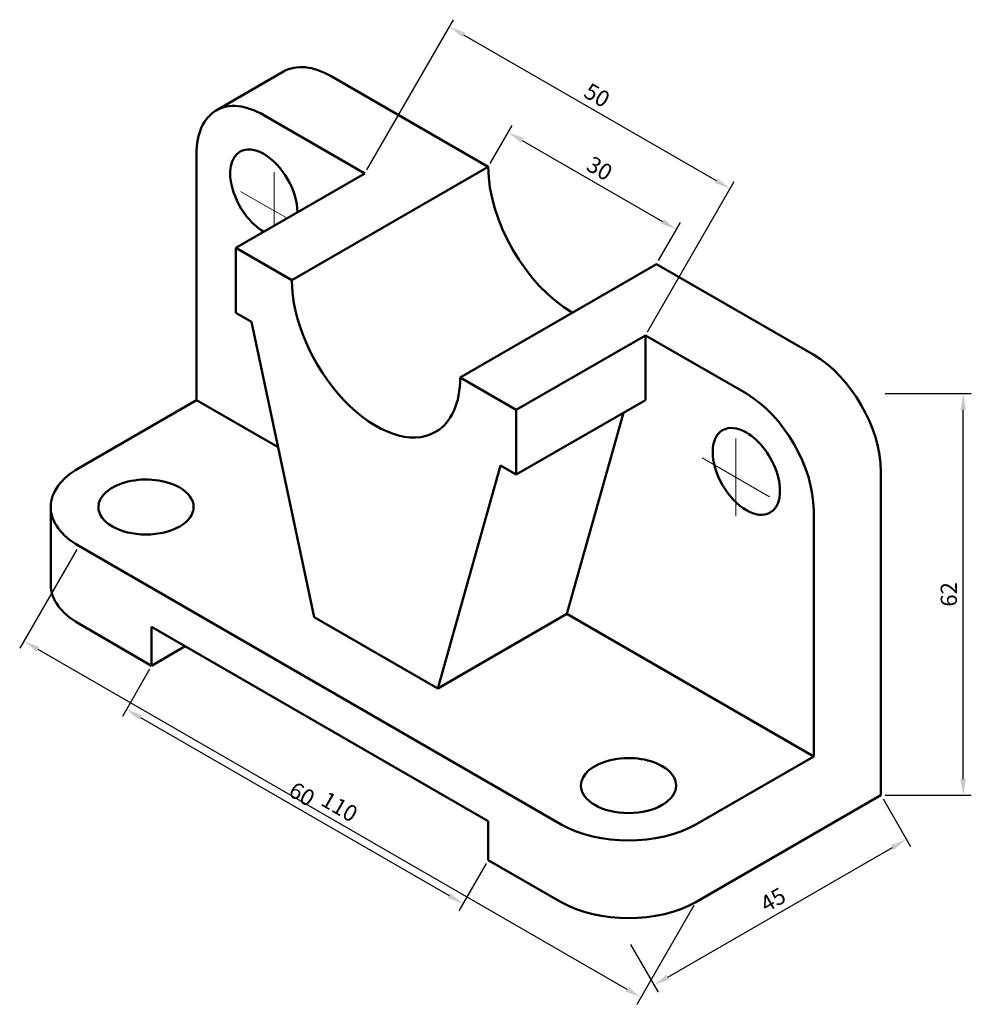
# Model space of a CAD drawing. Units: millimetres. Extents: x 1633 to 1780, y 2750 to 2902.
import ezdxf

# ---------------------------------------------------------------- set-up
doc = ezdxf.new("R2010")
doc.units = ezdxf.units.MM
doc.linetypes.add('CENTER', pattern=[50.8, 31.75, -6.35, 6.35, -6.35])
for name, color, linetype, lineweight in [('M-CNTR', 1, 'CENTER', 18), ('M-DIMS', 2, 'Continuous', 25), ('M-OUTL', 7, 'Continuous', 50)]:
    doc.layers.add(name, color=color, linetype=linetype, lineweight=lineweight)
doc.styles.get("Standard").update_dxf_attribs({"font": 'arial.ttf'})
doc.dimstyles.new('ISO-25', dxfattribs={"dimtxt": 2.5, "dimasz": 2.5, "dimexe": 1.25, "dimexo": 0.625, "dimtad": 1, "dimtxsty": 'Standard', "dimcen": 2.5, "dimadec": 0, "dimazin": 0, "dimtfac": 1, "dimtmove": 0, "dimatfit": 3, "dimfxl": 1, "dimarcsym": 0})

# ---------------------------------------------------------------- blocks, each defined once
blk = doc.blocks.new('*D1')
at = {"layer": 'Defpoints', "color": 0, "transparency": 16777216}
for p in [(1653.65, 2801.94), (1705.61, 2771.94), (1701.72, 2765.19)]:
    blk.add_point(p, dxfattribs=at)
at = {"layer": 'M-DIMS', "color": 0, "lineweight": -2, "transparency": 16777216}
for p, q in [((1653.33, 2801.4), (1649.13, 2794.11)), ((1651.92, 2793.94), (1699.55, 2766.44)), ((1705.3, 2771.4), (1701.09, 2764.11))]:
    blk.add_line(p, q, dxfattribs=at)
at = {"layer": 'M-DIMS', "color": 0, "transparency": 16777216}
for points in [[(1652.13, 2794.31), (1651.71, 2793.58), (1649.75, 2795.19)], [(1699.76, 2766.81), (1699.34, 2766.08), (1701.72, 2765.19)]]:
    blk.add_solid(points, dxfattribs=at)
at = {"layer": 'M-DIMS', "color": 0, "transparency": 16777216, "insert": (1676.69, 2781.84), "char_height": 2.5, "attachment_point": 5, "rotation": 330}
blk.add_mtext('60', dxfattribs=at)
blk = doc.blocks.new('*D2')
at = {"layer": 'Defpoints', "color": 0, "transparency": 16777216}
for p in [(1766.23, 2781.94), (1770.16, 2775.13), (1727.26, 2759.44)]:
    blk.add_point(p, dxfattribs=at)
at = {"layer": 'M-DIMS', "color": 0, "lineweight": -2, "transparency": 16777216}
for p, q in [((1766.54, 2781.4), (1770.78, 2774.05)), ((1733.35, 2753.88), (1767.99, 2773.88)), ((1727.57, 2758.9), (1731.81, 2751.55))]:
    blk.add_line(p, q, dxfattribs=at)
at = {"layer": 'M-DIMS', "color": 0, "transparency": 16777216}
for points in [[(1767.78, 2774.24), (1768.2, 2773.52), (1770.16, 2775.13)], [(1733.14, 2754.24), (1733.56, 2753.52), (1731.19, 2752.63)]]:
    blk.add_solid(points, dxfattribs=at)
at = {"layer": 'M-DIMS', "color": 0, "transparency": 16777216, "insert": (1749.72, 2765.53), "char_height": 2.5, "attachment_point": 5, "rotation": 30}
blk.add_mtext('45', dxfattribs=at)
blk = doc.blocks.new('*D3')
at = {"layer": 'Defpoints', "color": 0, "transparency": 16777216}
for p in [(1766.23, 2843.94), (1778.92, 2843.94), (1766.23, 2781.94)]:
    blk.add_point(p, dxfattribs=at)
at = {"layer": 'M-DIMS', "color": 0, "lineweight": -2, "transparency": 16777216}
for p, q in [((1766.86, 2843.94), (1780.17, 2843.94)), ((1778.92, 2784.44), (1778.92, 2841.44)), ((1766.86, 2781.94), (1780.17, 2781.94))]:
    blk.add_line(p, q, dxfattribs=at)
at = {"layer": 'M-DIMS', "color": 0, "transparency": 16777216}
for points in [[(1778.5, 2841.44), (1779.34, 2841.44), (1778.92, 2843.94)], [(1778.5, 2784.44), (1779.34, 2784.44), (1778.92, 2781.94)]]:
    blk.add_solid(points, dxfattribs=at)
at = {"layer": 'M-DIMS', "color": 0, "transparency": 16777216, "insert": (1777.02, 2812.94), "char_height": 2.5, "attachment_point": 5, "rotation": 90}
blk.add_mtext('62', dxfattribs=at)
blk = doc.blocks.new('*D4')
at = {"layer": 'Defpoints', "color": 0, "transparency": 16777216}
for p in [(1705.61, 2878.94), (1734.67, 2869.28), (1731.59, 2863.94)]:
    blk.add_point(p, dxfattribs=at)
at = {"layer": 'M-DIMS', "color": 0, "lineweight": -2, "transparency": 16777216}
for p, q in [((1705.92, 2879.48), (1709.32, 2885.36)), ((1710.86, 2883.03), (1732.51, 2870.53)), ((1731.9, 2864.48), (1735.3, 2870.36))]:
    blk.add_line(p, q, dxfattribs=at)
at = {"layer": 'M-DIMS', "color": 0, "transparency": 16777216}
for points in [[(1711.07, 2883.39), (1710.65, 2882.67), (1708.69, 2884.28)], [(1732.72, 2870.89), (1732.3, 2870.17), (1734.67, 2869.28)]]:
    blk.add_solid(points, dxfattribs=at)
at = {"layer": 'M-DIMS', "color": 0, "transparency": 16777216, "insert": (1722.63, 2878.43), "char_height": 2.5, "attachment_point": 5, "rotation": 330}
blk.add_mtext('30', dxfattribs=at)
blk = doc.blocks.new('*D5')
at = {"layer": 'Defpoints', "color": 0, "transparency": 16777216}
for p in [(1686.56, 2877.94), (1742.93, 2875.59), (1729.86, 2852.94)]:
    blk.add_point(p, dxfattribs=at)
at = {"layer": 'M-DIMS', "color": 0, "lineweight": -2, "transparency": 16777216}
for p, q in [((1686.87, 2878.48), (1700.26, 2901.67)), ((1701.8, 2899.34), (1740.77, 2876.84)), ((1730.17, 2853.48), (1743.56, 2876.67))]:
    blk.add_line(p, q, dxfattribs=at)
at = {"layer": 'M-DIMS', "color": 0, "transparency": 16777216}
for points in [[(1702.01, 2899.7), (1701.59, 2898.98), (1699.63, 2900.59)], [(1740.98, 2877.2), (1740.56, 2876.48), (1742.93, 2875.59)]]:
    blk.add_solid(points, dxfattribs=at)
at = {"layer": 'M-DIMS', "color": 0, "transparency": 16777216, "insert": (1722.23, 2889.73), "char_height": 2.5, "attachment_point": 5, "rotation": 330}
blk.add_mtext('50', dxfattribs=at)
blk = doc.blocks.new('*D7')
at = {"layer": 'Defpoints', "color": 0, "transparency": 16777216}
for p in [(1642.39, 2820.44), (1737.65, 2765.44), (1729.17, 2750.75)]:
    blk.add_point(p, dxfattribs=at)
at = {"layer": 'M-DIMS', "color": 0, "lineweight": -2, "transparency": 16777216}
for p, q in [((1642.08, 2819.9), (1633.28, 2804.66)), ((1636.07, 2804.5), (1727, 2752)), ((1737.34, 2764.9), (1728.54, 2749.66))]:
    blk.add_line(p, q, dxfattribs=at)
at = {"layer": 'M-DIMS', "color": 0, "transparency": 16777216}
for points in [[(1636.28, 2804.86), (1635.86, 2804.14), (1633.91, 2805.75)], [(1727.21, 2752.36), (1726.8, 2751.64), (1729.17, 2750.75)]]:
    blk.add_solid(points, dxfattribs=at)
at = {"layer": 'M-DIMS', "color": 0, "transparency": 16777216, "insert": (1682.49, 2779.89), "char_height": 2.5, "attachment_point": 5, "rotation": 330}
blk.add_mtext('110', dxfattribs=at)

msp = doc.modelspace()

# ---------------------------------------------------------------- linework, layer by layer
at = {"layer": 'M-CNTR'}
for p, q in [((1672.575, 2872.153), (1672.575, 2878.153)), ((1672.575, 2878.153), (1672.575, 2869.865)), ((1672.575, 2872.153), (1667.379, 2875.153)), ((1667.379, 2875.153), (1674.556, 2871.009)), ((1743.838, 2825.009), (1743.838, 2837.009)), ((1749.034, 2828.009), (1738.642, 2834.009)), ((1743.838, 2831.009), (1749.034, 2828.009)), ((1743.838, 2831.009), (1743.838, 2825.009))]:
    msp.add_line(p, q, dxfattribs=at)
at = {"layer": 'M-OUTL'}
for p, q in [((1663.619, 2887.665), (1674.011, 2893.665)), ((1705.608, 2878.937), (1681.36, 2892.937)), ((1686.556, 2877.937), (1670.967, 2886.937)), ((1660.575, 2842.937), (1660.575, 2880.937)), ((1666.637, 2866.437), (1686.556, 2877.937)), ((1675.297, 2861.437), (1705.608, 2878.937)), ((1666.637, 2866.437), (1675.297, 2861.437)), ((1666.637, 2856.437), (1666.637, 2866.437)), ((1701.278, 2846.437), (1731.589, 2863.937)), ((1755.838, 2849.937), (1731.589, 2863.937)), ((1669.062, 2855.037), (1666.637, 2856.437)), ((1678.761, 2809.437), (1669.062, 2855.037)), ((1709.938, 2841.437), (1729.857, 2852.937)), ((1729.857, 2852.937), (1729.857, 2852.937)), ((1745.445, 2843.937), (1729.857, 2852.937)), ((1729.857, 2842.937), (1729.857, 2852.937)), ((1701.278, 2846.437), (1709.938, 2841.437)), ((1642.388, 2832.437), (1660.575, 2842.937)), ((1673.184, 2835.657), (1660.575, 2842.937)), ((1709.938, 2831.437), (1729.857, 2842.937)), ((1709.938, 2831.437), (1709.938, 2841.437)), ((1726.489, 2840.993), (1717.733, 2809.937)), ((1707.513, 2832.837), (1697.814, 2798.437)), ((1709.938, 2831.437), (1707.513, 2832.837)), ((1766.23, 2781.937), (1766.23, 2831.937)), ((1638.084, 2814.437), (1638.084, 2826.437)), ((1755.838, 2787.937), (1755.838, 2825.937)), ((1716.867, 2777.437), (1642.388, 2820.437)), ((1697.814, 2798.437), (1678.761, 2809.437)), ((1697.814, 2798.437), (1717.733, 2809.937)), ((1755.838, 2787.937), (1717.733, 2809.937)), ((1653.647, 2801.937), (1642.388, 2808.437)), ((1653.647, 2801.937), (1653.647, 2807.937)), ((1705.608, 2777.937), (1653.647, 2807.937)), ((1653.647, 2801.937), (1658.843, 2804.937)), ((1737.651, 2777.437), (1755.838, 2787.937)), ((1737.651, 2765.437), (1766.23, 2781.937)), ((1705.608, 2771.937), (1705.608, 2777.937)), ((1716.867, 2765.437), (1705.608, 2771.937))]:
    msp.add_line(p, q, dxfattribs=at)
for centre, major_axis, start_param, end_param in [((1681.36, 2880.937), (-7.348, 12.728), 5.4977871, 6.2831853), ((1670.967, 2874.937), (-7.348, 12.728), 5.4977871, 6.2831853), ((1670.967, 2874.937), (-7.348, 12.728), 0, 0.7853982), ((1670.967, 2874.937), (3.674, -6.364), 3.1415927, 5.4977871), ((1670.967, 2874.937), (3.674, -6.364), 2.3561945, 3.1415927), ((1670.967, 2874.937), (3.674, -6.364), 0.7853982, 2.3561945), ((1718.599, 2871.437), (9.186, -15.91), 3.9269908, 5.4977871), ((1688.288, 2853.937), (9.186, -15.91), 3.9269908, 6.2831853), ((1755.838, 2837.937), (7.348, -12.728), 0.7853982, 2.3561945), ((1688.288, 2853.937), (9.186, -15.91), 0, 0.7853982), ((1745.445, 2831.937), (7.348, -12.728), 0.7853982, 2.3561945), ((1745.445, 2831.937), (3.674, -6.364), 3.1415927, 6.2831853), ((1745.445, 2831.937), (3.674, -6.364), 2.3561945, 3.1415927), ((1745.445, 2831.937), (3.674, -6.364), 0, 2.3561945), ((1652.781, 2826.437), (-14.697, 0), 5.4977871, 6.2831853), ((1652.781, 2826.437), (7.348, 0), 0.7853982, 3.1415927), ((1652.781, 2826.437), (7.348, 0), 0, 0.7853982), ((1652.781, 2826.437), (-14.697, 0), 0, 0.7853982), ((1652.781, 2826.437), (7.348, 0), 3.1415927, 6.2831853), ((1652.781, 2814.437), (-14.697, 0), 0, 0.7853982), ((1727.259, 2783.437), (7.348, 0), 0.7853982, 3.1415927), ((1727.259, 2783.437), (7.348, 0), 0, 0.7853982), ((1727.259, 2783.437), (7.348, 0), 3.1415927, 6.2831853), ((1727.259, 2783.437), (14.697, 0), 3.9269908, 5.4977871), ((1727.259, 2771.437), (14.697, 0), 3.9269908, 5.4977871)]:
    msp.add_ellipse(centre, major_axis=major_axis, ratio=0.5773503, start_param=start_param, end_param=end_param, dxfattribs=at)

# ---------------------------------------------------------------- dimensions: what is measured, and where the dimension line sits
at = {"layer": 'M-DIMS'}
for p1, p2, distance, picture, middle in [((1686.556, 2877.937), (1729.857, 2852.937), 26.155, '*D5', (1722.235, 2889.735)), ((1705.608, 2878.937), (1731.589, 2863.937), 6.168, '*D4', (1722.634, 2878.426)), ((1766.23, 2781.937), (1766.23, 2843.937), -12.689, '*D3', (1777.018, 2812.937)), ((1653.647, 2801.937), (1705.608, 2771.937), -7.785, '*D1', (1676.686, 2781.842)), ((1727.259, 2759.437), (1766.23, 2781.937), -7.856, '*D2', (1749.724, 2765.526))]:
    dim = msp.add_aligned_dim(p1=p1, p2=p2, distance=distance, dimstyle='ISO-25', override={"dimclrd": 0, "dimclre": 0, "dimclrt": 0}, dxfattribs=at)
    dim.commit()
    dim.dimension.update_dxf_attribs({"geometry": picture, "text_midpoint": middle})
dim = msp.add_linear_dim(base=(1729.17, 2750.747), p1=(1642.388, 2820.437), p2=(1737.651, 2765.437), angle=330, dimstyle='ISO-25', override={"dimrnd": 0}, dxfattribs=at)
dim.commit()
dim.dimension.update_dxf_attribs({"geometry": '*D7', "text_midpoint": (1682.489, 2779.894)})

doc.saveas('drawing.dxf')
